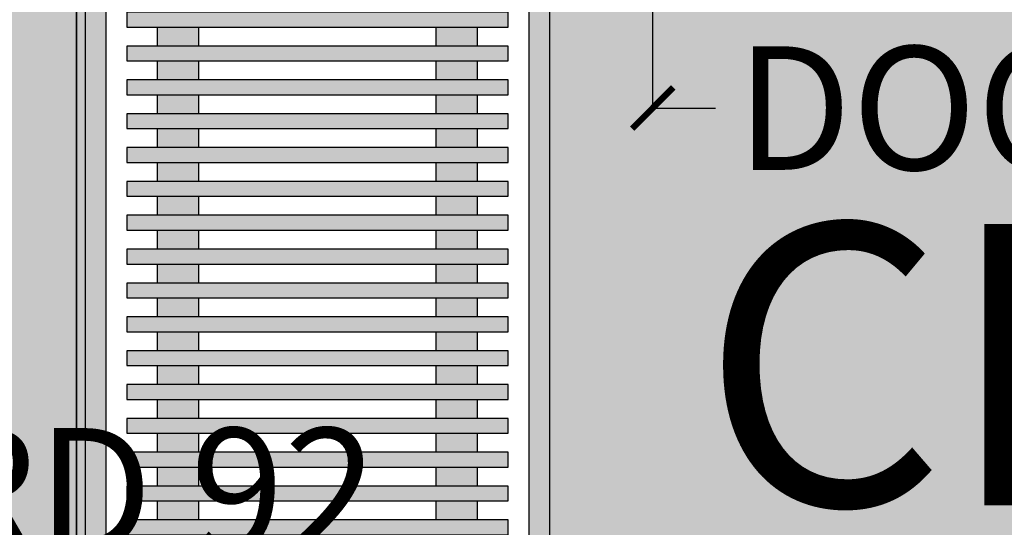
# Model space of a CAD drawing. Units: inches. Extents: x 1704 to 6393, y -157 to 1172.
# Tile 30 of 122: x 2351 to 2398, y 316 to 341. Entities that reach past the tile are written whole.
import ezdxf

# ---------------------------------------------------------------- set-up
doc = ezdxf.new("R2010")
doc.units = ezdxf.units.IN
doc.header["$MEASUREMENT"] = 0
for name, color, linetype, lineweight in [('A-ANNO-DIMS', 7, 'Continuous', 13), ('A-AREA-IDEN', 7, 'Continuous', 18), ('A-FURN', 8, 'Continuous', 18), ('A-WALL-PATT', 7, 'Continuous', 13), ('estofado', 7, 'Continuous', 25), ('WALLS', 7, 'Continuous', 35)]:
    doc.layers.add(name, color=color, linetype=linetype, lineweight=lineweight)
doc.layers.add('A-FLOR-PATT', color=7, linetype='Continuous', lineweight=13, true_color=0xf2f2f2)
doc.layers.add('MOBIL', color=7, linetype='Continuous')
doc.styles.get("Standard").update_dxf_attribs({"font": 'arial.ttf'})
doc.dimstyles.get("Standard").update_dxf_attribs({"dimtxt": 6, "dimasz": 2, "dimexe": 0.18, "dimexo": 0.0625, "dimgap": 0.09, "dimtad": 0, "dimtih": 1, "dimtoh": 1, "dimdec": 1, "dimzin": 0, "dimdsep": 46, "dimlunit": 3, "dimtxsty": 'Standard', "dimblk": 'ARCHTICK', "dimcen": 0.09, "dimadec": 0, "dimazin": 0, "dimtfac": 1, "dimtdec": 1, "dimtofl": 0, "dimtmove": 0, "dimatfit": 3, "dimfxl": 1, "dimtolj": 1, "dimtzin": 0, "dimarcsym": 0})

# ---------------------------------------------------------------- blocks, each defined once
blk = doc.blocks.new('Aparador Aido WV')
at = {"layer": 'MOBIL'}
h = blk.add_hatch(color=256, dxfattribs=at)
h.set_gradient(color1=(226, 228, 228), one_color=1, tint=1, name='CYLINDER')
h.paths.add_polyline_path([(0.9, -0.02), (0.9, 0), (-0.9, 0), (-0.9, -0.02)])
h = blk.add_hatch(color=256, dxfattribs=at)
h.set_gradient(color1=(106, 79, 62), color2=(55, 41, 32), one_color=1, tint=0.17)
h.paths.add_polyline_path([(-0.04342, -0.04017), (-0.04342, -0.40983), (-0.02906, -0.40983), (-0.02906, -0.04017)])
h = blk.add_hatch(color=256, dxfattribs=at)
h.set_gradient(color1=(106, 79, 62), color2=(55, 41, 32), one_color=1, tint=0.17)
h.paths.add_polyline_path([(-0.01067, -0.04017), (-0.01067, -0.40983), (0.00369, -0.40983), (0.00369, -0.04017)])
h = blk.add_hatch(color=256, dxfattribs=at)
h.set_gradient(color1=(106, 79, 62), color2=(55, 41, 32), one_color=1, tint=0.17)
h.paths.add_polyline_path([(0.02208, -0.04017), (0.02208, -0.40983), (0.03644, -0.40983), (0.03644, -0.04017)])
h = blk.add_hatch(color=256, dxfattribs=at)
h.set_gradient(color1=(106, 79, 62), color2=(55, 41, 32), one_color=1, tint=0.17)
h.paths.add_polyline_path([(0.05483, -0.04017), (0.05483, -0.40983), (0.0692, -0.40983), (0.0692, -0.04017)])
h = blk.add_hatch(color=256, dxfattribs=at)
h.set_gradient(color1=(106, 79, 62), color2=(55, 41, 32), one_color=1, tint=0.17)
h.paths.add_polyline_path([(0.10195, -0.04017), (0.08758, -0.04017), (0.08758, -0.40983), (0.10195, -0.40983)])
h = blk.add_hatch(color=256, dxfattribs=at)
h.set_gradient(color1=(106, 79, 62), color2=(55, 41, 32), one_color=1, tint=0.17)
h.paths.add_polyline_path([(0.12033, -0.04017), (0.12033, -0.40983), (0.1347, -0.40983), (0.1347, -0.04017)])
h = blk.add_hatch(color=256, dxfattribs=at)
h.set_gradient(color1=(106, 79, 62), color2=(55, 41, 32), one_color=1, tint=0.17)
h.paths.add_polyline_path([(0.15309, -0.04017), (0.15309, -0.40983), (0.16745, -0.40983), (0.16745, -0.04017)])
h = blk.add_hatch(color=256, dxfattribs=at)
h.set_gradient(color1=(106, 79, 62), color2=(55, 41, 32), one_color=1, tint=0.17)
h.paths.add_polyline_path([(0.18584, -0.04017), (0.18584, -0.40983), (0.2002, -0.40983), (0.2002, -0.04017)])
h = blk.add_hatch(color=256, dxfattribs=at)
h.set_gradient(color1=(106, 79, 62), color2=(55, 41, 32), one_color=1, tint=0.17)
h.paths.add_polyline_path([(0.21859, -0.04017), (0.21859, -0.40983), (0.23295, -0.40983), (0.23295, -0.04017)])
h = blk.add_hatch(color=256, dxfattribs=at)
h.set_gradient(color1=(106, 79, 62), color2=(55, 41, 32), one_color=1, tint=0.17)
h.paths.add_polyline_path([(0.25134, -0.04017), (0.25134, -0.40983), (0.26571, -0.40983), (0.26571, -0.04017)])
h = blk.add_hatch(color=256, dxfattribs=at)
h.set_gradient(color1=(106, 79, 62), color2=(55, 41, 32), one_color=1, tint=0.17)
h.paths.add_polyline_path([(0.28409, -0.04017), (0.28409, -0.40983), (0.29846, -0.40983), (0.29846, -0.04017)])
h = blk.add_hatch(color=256, dxfattribs=at)
h.set_gradient(color1=(106, 79, 62), color2=(55, 41, 32), one_color=1, tint=0.17)
h.paths.add_polyline_path([(0.31684, -0.04017), (0.31684, -0.40983), (0.33121, -0.40983), (0.33121, -0.04017)])
h = blk.add_hatch(color=256, dxfattribs=at)
h.set_gradient(color1=(106, 79, 62), color2=(55, 41, 32), one_color=1, tint=0.17)
h.paths.add_polyline_path([(0.3496, -0.04017), (0.3496, -0.40983), (0.36396, -0.40983), (0.36396, -0.04017)])
h = blk.add_hatch(color=256, dxfattribs=at)
h.set_gradient(color1=(106, 79, 62), color2=(55, 41, 32), one_color=1, tint=0.17)
h.paths.add_polyline_path([(0.38235, -0.04017), (0.38235, -0.40983), (0.39671, -0.40983), (0.39671, -0.04017)])
h = blk.add_hatch(color=256, dxfattribs=at)
h.set_gradient(color1=(106, 79, 62), color2=(55, 41, 32), one_color=1, tint=0.17)
h.paths.add_polyline_path([(0.4151, -0.40983), (0.42946, -0.40983), (0.42946, -0.04017), (0.4151, -0.04017)])
h = blk.add_hatch(color=256, dxfattribs=at)
h.set_gradient(color1=(106, 79, 62), color2=(55, 41, 32), one_color=1, tint=0.17)
h.paths.add_polyline_path([(0.44785, -0.04017), (0.44785, -0.40983), (0.46222, -0.40983), (0.46222, -0.04017)])
h = blk.add_hatch(color=256, dxfattribs=at)
h.set_gradient(color1=(106, 79, 62), color2=(157, 117, 92), one_color=1, tint=0.49)
h.paths.add_polyline_path([(-0.01067, -0.07), (-0.02906, -0.07), (-0.02906, -0.11), (-0.01067, -0.11)])
h = blk.add_hatch(color=256, dxfattribs=at)
h.set_gradient(color1=(106, 79, 62), color2=(157, 117, 92), one_color=1, tint=0.49)
h.paths.add_polyline_path([(0.02208, -0.07), (0.00369, -0.07), (0.00369, -0.11), (0.02208, -0.11)])
h = blk.add_hatch(color=256, dxfattribs=at)
h.set_gradient(color1=(106, 79, 62), color2=(157, 117, 92), one_color=1, tint=0.49)
h.paths.add_polyline_path([(0.05483, -0.07), (0.03644, -0.07), (0.03644, -0.11), (0.05483, -0.11)])
h = blk.add_hatch(color=256, dxfattribs=at)
h.set_gradient(color1=(106, 79, 62), color2=(157, 117, 92), one_color=1, tint=0.49)
h.paths.add_polyline_path([(0.08758, -0.07), (0.0692, -0.07), (0.0692, -0.11), (0.08758, -0.11)])
h = blk.add_hatch(color=256, dxfattribs=at)
h.set_gradient(color1=(106, 79, 62), color2=(157, 117, 92), one_color=1, tint=0.49)
h.paths.add_polyline_path([(0.12033, -0.07), (0.10195, -0.07), (0.10195, -0.11), (0.12033, -0.11)])
h = blk.add_hatch(color=256, dxfattribs=at)
h.set_gradient(color1=(106, 79, 62), color2=(157, 117, 92), one_color=1, tint=0.49)
h.paths.add_polyline_path([(0.15309, -0.07), (0.1347, -0.07), (0.1347, -0.11), (0.15309, -0.11)])
h = blk.add_hatch(color=256, dxfattribs=at)
h.set_gradient(color1=(106, 79, 62), color2=(157, 117, 92), one_color=1, tint=0.49)
h.paths.add_polyline_path([(0.18584, -0.07), (0.16745, -0.07), (0.16745, -0.11), (0.18584, -0.11)])
h = blk.add_hatch(color=256, dxfattribs=at)
h.set_gradient(color1=(106, 79, 62), color2=(157, 117, 92), one_color=1, tint=0.49)
h.paths.add_polyline_path([(0.21859, -0.07), (0.2002, -0.07), (0.2002, -0.11), (0.21859, -0.11)])
h = blk.add_hatch(color=256, dxfattribs=at)
h.set_gradient(color1=(106, 79, 62), color2=(157, 117, 92), one_color=1, tint=0.49)
h.paths.add_polyline_path([(0.25134, -0.07), (0.23295, -0.07), (0.23295, -0.11), (0.25134, -0.11)])
h = blk.add_hatch(color=256, dxfattribs=at)
h.set_gradient(color1=(106, 79, 62), color2=(157, 117, 92), one_color=1, tint=0.49)
h.paths.add_polyline_path([(0.28409, -0.07), (0.26571, -0.07), (0.26571, -0.11), (0.28409, -0.11)])
h = blk.add_hatch(color=256, dxfattribs=at)
h.set_gradient(color1=(106, 79, 62), color2=(157, 117, 92), one_color=1, tint=0.49)
h.paths.add_polyline_path([(0.31684, -0.07), (0.29846, -0.07), (0.29846, -0.11), (0.31684, -0.11)])
h = blk.add_hatch(color=256, dxfattribs=at)
h.set_gradient(color1=(106, 79, 62), color2=(157, 117, 92), one_color=1, tint=0.49)
h.paths.add_polyline_path([(0.3496, -0.07), (0.33121, -0.07), (0.33121, -0.11), (0.3496, -0.11)])
h = blk.add_hatch(color=256, dxfattribs=at)
h.set_gradient(color1=(106, 79, 62), color2=(157, 117, 92), one_color=1, tint=0.49)
h.paths.add_polyline_path([(0.38235, -0.07), (0.36396, -0.07), (0.36396, -0.11), (0.38235, -0.11)])
h = blk.add_hatch(color=256, dxfattribs=at)
h.set_gradient(color1=(106, 79, 62), color2=(157, 117, 92), one_color=1, tint=0.49)
h.paths.add_polyline_path([(0.4151, -0.07), (0.39671, -0.07), (0.39671, -0.11), (0.4151, -0.11)])
h = blk.add_hatch(color=256, dxfattribs=at)
h.set_gradient(color1=(106, 79, 62), color2=(157, 117, 92), one_color=1, tint=0.49)
h.paths.add_polyline_path([(0.44785, -0.07), (0.42946, -0.07), (0.42946, -0.11), (0.44785, -0.11)])
h = blk.add_hatch(color=256, dxfattribs=at)
h.set_gradient(color1=(106, 79, 62), color2=(157, 117, 92), one_color=1, tint=0.49)
h.paths.add_polyline_path([(-0.01067, -0.34), (-0.02906, -0.34), (-0.02906, -0.38), (-0.01067, -0.38)])
h = blk.add_hatch(color=256, dxfattribs=at)
h.set_gradient(color1=(106, 79, 62), color2=(157, 117, 92), one_color=1, tint=0.49)
h.paths.add_polyline_path([(0.02208, -0.34), (0.00369, -0.34), (0.00369, -0.38), (0.02208, -0.38)])
h = blk.add_hatch(color=256, dxfattribs=at)
h.set_gradient(color1=(106, 79, 62), color2=(157, 117, 92), one_color=1, tint=0.49)
h.paths.add_polyline_path([(0.05483, -0.34), (0.03644, -0.34), (0.03644, -0.38), (0.05483, -0.38)])
h = blk.add_hatch(color=256, dxfattribs=at)
h.set_gradient(color1=(106, 79, 62), color2=(157, 117, 92), one_color=1, tint=0.49)
h.paths.add_polyline_path([(0.08758, -0.34), (0.0692, -0.34), (0.0692, -0.38), (0.08758, -0.38)])
h = blk.add_hatch(color=256, dxfattribs=at)
h.set_gradient(color1=(106, 79, 62), color2=(157, 117, 92), one_color=1, tint=0.49)
h.paths.add_polyline_path([(0.12033, -0.34), (0.10195, -0.34), (0.10195, -0.38), (0.12033, -0.38)])
h = blk.add_hatch(color=256, dxfattribs=at)
h.set_gradient(color1=(106, 79, 62), color2=(157, 117, 92), one_color=1, tint=0.49)
h.paths.add_polyline_path([(0.15309, -0.34), (0.1347, -0.34), (0.1347, -0.38), (0.15309, -0.38)])
h = blk.add_hatch(color=256, dxfattribs=at)
h.set_gradient(color1=(106, 79, 62), color2=(157, 117, 92), one_color=1, tint=0.49)
h.paths.add_polyline_path([(0.18584, -0.34), (0.16745, -0.34), (0.16745, -0.38), (0.18584, -0.38)])
h = blk.add_hatch(color=256, dxfattribs=at)
h.set_gradient(color1=(106, 79, 62), color2=(157, 117, 92), one_color=1, tint=0.49)
h.paths.add_polyline_path([(0.21859, -0.34), (0.2002, -0.34), (0.2002, -0.38), (0.21859, -0.38)])
h = blk.add_hatch(color=256, dxfattribs=at)
h.set_gradient(color1=(106, 79, 62), color2=(157, 117, 92), one_color=1, tint=0.49)
h.paths.add_polyline_path([(0.25134, -0.34), (0.23295, -0.34), (0.23295, -0.38), (0.25134, -0.38)])
h = blk.add_hatch(color=256, dxfattribs=at)
h.set_gradient(color1=(106, 79, 62), color2=(157, 117, 92), one_color=1, tint=0.49)
h.paths.add_polyline_path([(0.28409, -0.34), (0.26571, -0.34), (0.26571, -0.38), (0.28409, -0.38)])
h = blk.add_hatch(color=256, dxfattribs=at)
h.set_gradient(color1=(106, 79, 62), color2=(157, 117, 92), one_color=1, tint=0.49)
h.paths.add_polyline_path([(0.31684, -0.34), (0.29846, -0.34), (0.29846, -0.38), (0.31684, -0.38)])
h = blk.add_hatch(color=256, dxfattribs=at)
h.set_gradient(color1=(106, 79, 62), color2=(157, 117, 92), one_color=1, tint=0.49)
h.paths.add_polyline_path([(0.3496, -0.34), (0.33121, -0.34), (0.33121, -0.38), (0.3496, -0.38)])
h = blk.add_hatch(color=256, dxfattribs=at)
h.set_gradient(color1=(106, 79, 62), color2=(157, 117, 92), one_color=1, tint=0.49)
h.paths.add_polyline_path([(0.38235, -0.34), (0.36396, -0.34), (0.36396, -0.38), (0.38235, -0.38)])
h = blk.add_hatch(color=256, dxfattribs=at)
h.set_gradient(color1=(106, 79, 62), color2=(157, 117, 92), one_color=1, tint=0.49)
h.paths.add_polyline_path([(0.4151, -0.34), (0.39671, -0.34), (0.39671, -0.38), (0.4151, -0.38)])
h = blk.add_hatch(color=256, dxfattribs=at)
h.set_gradient(color1=(106, 79, 62), color2=(157, 117, 92), one_color=1, tint=0.49)
h.paths.add_polyline_path([(0.44785, -0.34), (0.42946, -0.34), (0.42946, -0.38), (0.44785, -0.38)])
h = blk.add_hatch(color=256, dxfattribs=at)
h.set_gradient(color1=(226, 228, 228), one_color=1, tint=1, name='CYLINDER')
h.paths.add_polyline_path([(0.9, -0.45), (0.9, -0.43), (-0.9, -0.43), (-0.9, -0.45)])
at = {"layer": 'estofado', "ltscale": 0.5}
for p, q in [((-0.02906, -0.07), (-0.01067, -0.07)), ((0.00369, -0.07), (0.02208, -0.07)), ((0.03644, -0.07), (0.05483, -0.07)), ((0.0692, -0.07), (0.08758, -0.07)), ((0.10195, -0.07), (0.12033, -0.07)), ((0.1347, -0.07), (0.15309, -0.07)), ((0.16745, -0.07), (0.18584, -0.07)), ((0.2002, -0.07), (0.21859, -0.07)), ((0.23295, -0.07), (0.25134, -0.07)), ((0.26571, -0.07), (0.28409, -0.07)), ((0.29846, -0.07), (0.31684, -0.07)), ((0.33121, -0.07), (0.3496, -0.07)), ((0.36396, -0.07), (0.38235, -0.07)), ((0.39671, -0.07), (0.4151, -0.07)), ((0.42946, -0.07), (0.44785, -0.07)), ((-0.02906, -0.11), (-0.01067, -0.11)), ((0.00369, -0.11), (0.02208, -0.11)), ((0.03644, -0.11), (0.05483, -0.11)), ((0.0692, -0.11), (0.08758, -0.11)), ((0.10195, -0.11), (0.12033, -0.11)), ((0.1347, -0.11), (0.15309, -0.11)), ((0.16745, -0.11), (0.18584, -0.11)), ((0.2002, -0.11), (0.21859, -0.11)), ((0.23295, -0.11), (0.25134, -0.11)), ((0.26571, -0.11), (0.28409, -0.11)), ((0.29846, -0.11), (0.31684, -0.11)), ((0.33121, -0.11), (0.3496, -0.11)), ((0.36396, -0.11), (0.38235, -0.11)), ((0.39671, -0.11), (0.4151, -0.11)), ((0.42946, -0.11), (0.44785, -0.11)), ((-0.02906, -0.34), (-0.01067, -0.34)), ((0.00369, -0.34), (0.02208, -0.34)), ((0.03644, -0.34), (0.05483, -0.34)), ((0.0692, -0.34), (0.08758, -0.34)), ((0.10195, -0.34), (0.12033, -0.34)), ((0.1347, -0.34), (0.15309, -0.34)), ((0.16745, -0.34), (0.18584, -0.34)), ((0.2002, -0.34), (0.21859, -0.34)), ((0.23295, -0.34), (0.25134, -0.34)), ((0.26571, -0.34), (0.28409, -0.34)), ((0.29846, -0.34), (0.31684, -0.34)), ((0.33121, -0.34), (0.3496, -0.34)), ((0.36396, -0.34), (0.38235, -0.34)), ((0.39671, -0.34), (0.4151, -0.34)), ((0.42946, -0.34), (0.44785, -0.34)), ((-0.02906, -0.38), (-0.01067, -0.38)), ((0.00369, -0.38), (0.02208, -0.38)), ((0.03644, -0.38), (0.05483, -0.38)), ((0.0692, -0.38), (0.08758, -0.38)), ((0.10195, -0.38), (0.12033, -0.38)), ((0.1347, -0.38), (0.15309, -0.38)), ((0.16745, -0.38), (0.18584, -0.38)), ((0.2002, -0.38), (0.21859, -0.38)), ((0.23295, -0.38), (0.25134, -0.38)), ((0.26571, -0.38), (0.28409, -0.38)), ((0.29846, -0.38), (0.31684, -0.38)), ((0.33121, -0.38), (0.3496, -0.38)), ((0.36396, -0.38), (0.38235, -0.38)), ((0.39671, -0.38), (0.4151, -0.38)), ((0.42946, -0.38), (0.44785, -0.38))]:
    blk.add_line(p, q, dxfattribs=at)
for points in [[(-0.04342, -0.04017), (-0.04342, -0.40983), (-0.02906, -0.40983), (-0.02906, -0.04017)], [(-0.01067, -0.04017), (-0.01067, -0.40983), (0.00369, -0.40983), (0.00369, -0.04017)], [(0.02208, -0.04017), (0.02208, -0.40983), (0.03644, -0.40983), (0.03644, -0.04017)], [(0.05483, -0.04017), (0.05483, -0.40983), (0.0692, -0.40983), (0.0692, -0.04017)], [(0.08758, -0.04017), (0.08758, -0.40983), (0.10195, -0.40983), (0.10195, -0.04017)], [(0.12033, -0.04017), (0.12033, -0.40983), (0.1347, -0.40983), (0.1347, -0.04017)], [(0.15309, -0.04017), (0.15309, -0.40983), (0.16745, -0.40983), (0.16745, -0.04017)], [(0.18584, -0.04017), (0.18584, -0.40983), (0.2002, -0.40983), (0.2002, -0.04017)], [(0.21859, -0.04017), (0.21859, -0.40983), (0.23295, -0.40983), (0.23295, -0.04017)], [(0.25134, -0.04017), (0.25134, -0.40983), (0.26571, -0.40983), (0.26571, -0.04017)], [(0.28409, -0.04017), (0.28409, -0.40983), (0.29846, -0.40983), (0.29846, -0.04017)], [(0.31684, -0.04017), (0.31684, -0.40983), (0.33121, -0.40983), (0.33121, -0.04017)], [(0.3496, -0.04017), (0.3496, -0.40983), (0.36396, -0.40983), (0.36396, -0.04017)], [(0.38235, -0.04017), (0.38235, -0.40983), (0.39671, -0.40983), (0.39671, -0.04017)], [(0.4151, -0.04017), (0.4151, -0.40983), (0.42946, -0.40983), (0.42946, -0.04017)], [(0.44785, -0.04017), (0.44785, -0.40983), (0.46222, -0.40983), (0.46222, -0.04017)]]:
    blk.add_lwpolyline(points, close=True, dxfattribs=at)
at = {"layer": 'MOBIL'}
for p, q in [((0.9, -0.02), (-0.9, -0.02)), ((-0.9, -0.43), (0.9, -0.43))]:
    blk.add_line(p, q, dxfattribs=at)
blk.add_lwpolyline([(-0.9, -0.45), (0.9, -0.45), (0.9, 0), (-0.9, 0)], close=True, dxfattribs=at)
blk = doc.blocks.new('_ArchTick')
at = {"color": 0, "linetype": 'ByBlock', "const_width": 0.15}
blk.add_lwpolyline([(-0.5, -0.5), (0.5, 0.5)], dxfattribs=at)
blk = doc.blocks.new('*D30')
at = {"layer": 'A-ANNO-DIMS', "color": 0, "lineweight": -2, "transparency": 16777216}
for p, q in [((2381.349, 342.693), (2381.349, 336.276)), ((2423.349, 342.693), (2423.349, 336.276)), ((2381.349, 336.456), (2384.404, 336.456)), ((2423.349, 336.456), (2420.293, 336.456))]:
    blk.add_line(p, q, dxfattribs=at)
at = {"layer": 'Defpoints', "color": 0, "lineweight": -3, "transparency": 16777216}
for p in [(2381.349, 342.756), (2423.349, 342.756), (2423.349, 336.456)]:
    blk.add_point(p, dxfattribs=at)
at = {"layer": 'A-ANNO-DIMS', "color": 0, "lineweight": -2, "transparency": 16777216, "xscale": 2, "yscale": 2, "zscale": 2, "rotation": 180}
blk.add_blockref('_ArchTick', (2381.349, 336.456), dxfattribs=at)
at = {"layer": 'A-ANNO-DIMS', "color": 0, "lineweight": -2, "transparency": 16777216, "xscale": 2, "yscale": 2, "zscale": 2}
blk.add_blockref('_ArchTick', (2423.349, 336.456), dxfattribs=at)
at = {"layer": 'A-ANNO-DIMS', "color": 0, "transparency": 16777216, "insert": (2402.349, 336.456), "char_height": 6, "attachment_point": 5}
blk.add_mtext('\\A1;DOOR 42', dxfattribs=at)
blk = doc.blocks.new('*D68')
at = {"layer": 'A-ANNO-DIMS', "color": 0, "lineweight": -2, "transparency": 16777216}
for p, q in [((2353.706, 363.767), (2339.834, 363.767)), ((2340.014, 363.767), (2340.014, 321.111)), ((2340.014, 272.066), (2340.014, 314.722)), ((2353.706, 272.066), (2339.834, 272.066))]:
    blk.add_line(p, q, dxfattribs=at)
at = {"layer": 'Defpoints', "color": 0, "lineweight": -3, "transparency": 16777216}
for p in [(2340.014, 363.767), (2353.769, 363.767), (2353.769, 272.066)]:
    blk.add_point(p, dxfattribs=at)
at = {"layer": 'A-ANNO-DIMS', "color": 0, "lineweight": -2, "transparency": 16777216, "xscale": 2, "yscale": 2, "zscale": 2}
for p, rotation in [((2340.014, 363.767), 90), ((2340.014, 272.066), 270)]:
    blk.add_blockref('_ArchTick', p, dxfattribs=dict(at, rotation=rotation))
at = {"layer": 'A-ANNO-DIMS', "color": 0, "transparency": 16777216, "insert": (2340.014, 317.916), "char_height": 6, "attachment_point": 5}
blk.add_mtext('\\A1;SIDEBOARD 92', dxfattribs=at)
blk = doc.blocks.new('*D93')
at = {"layer": 'A-ANNO-DIMS', "color": 0, "lineweight": -2, "transparency": 16777216}
for p, q in [((2605.286, 895.213), (1829.698, 895.213)), ((1829.878, 895.213), (1829.878, 495.866)), ((1829.878, 90.213), (1829.878, 489.56)), ((2605.286, 90.213), (1829.698, 90.213))]:
    blk.add_line(p, q, dxfattribs=at)
at = {"layer": 'Defpoints', "color": 0, "lineweight": -3, "transparency": 16777216}
for p in [(2605.349, 895.213), (1829.878, 90.213), (2605.349, 90.213)]:
    blk.add_point(p, dxfattribs=at)
at = {"layer": 'A-ANNO-DIMS', "color": 0, "lineweight": -2, "transparency": 16777216, "xscale": 2, "yscale": 2, "zscale": 2}
for p, rotation in [((1829.878, 895.213), 90), ((1829.878, 90.213), 270)]:
    blk.add_blockref('_ArchTick', p, dxfattribs=dict(at, rotation=rotation))
at = {"layer": 'A-ANNO-DIMS', "color": 0, "transparency": 16777216, "insert": (1829.878, 492.713), "char_height": 6, "attachment_point": 5}
blk.add_mtext('\\A1;805', dxfattribs=at)

msp = doc.modelspace()

# ---------------------------------------------------------------- hatches: boundary and pattern name
at = {"layer": 'A-FLOR-PATT', "transparency": 33554528}
h = msp.add_hatch(color=256, dxfattribs=at)
h.dxf.hatch_style = 1
h.paths.add_polyline_path([(2325.349, 863.213), (2325.349, 887.213), (2263.349, 887.213), (2167.349, 887.213), (2081.349, 887.213), (2081.349, 719.213), (2277.349, 719.213), (2277.349, 711.213), (2277.349, 372.213), (2349.349, 372.213), (2381.349, 372.213), (2381.349, 364.213), (2353.349, 364.213), (2353.349, 270.213), (2381.349, 270.213), (2381.349, 266.213), (2357.349, 266.213), (2357.349, 98.213), (2381.349, 98.213), (2385.181, 98.213), (2386.482, 98.213), (2424.215, 98.213), (2425.516, 98.213), (2429.349, 98.213), (2597.349, 98.213), (2597.349, 146.213), (2597.349, 218.213), (2597.349, 266.213), (2423.349, 266.213), (2423.349, 270.213), (2473.349, 270.213), (2473.349, 294.213), (2477.349, 294.213), (2477.349, 270.213), (2547.349, 270.213), (2547.349, 364.213), (2477.349, 364.213), (2477.349, 318.213), (2473.349, 318.213), (2473.349, 364.213), (2423.349, 364.213), (2423.349, 372.213), (2469.349, 372.213), (2469.349, 459.213), (2469.349, 538.213), (2350.349, 538.213), (2350.349, 565.713), (2358.349, 565.713), (2358.349, 545.213), (2420.349, 545.213), (2420.349, 610.213), (2358.349, 610.213), (2358.349, 589.713), (2350.349, 589.713), (2350.349, 615.213), (2425.349, 615.213), (2425.349, 607.213), (2425.349, 546.213), (2469.349, 546.213), (2514.349, 546.213), (2514.349, 607.213), (2449.349, 607.213), (2449.349, 615.213), (2451.738, 615.213), (2451.738, 659.213), (2427.738, 659.213), (2427.738, 665.213), (2367.738, 665.213), (2367.738, 667.213), (2367.738, 711.213), (2325.349, 711.213), (2325.349, 719.213), (2325.349, 755.213), (2325.349, 763.213)])
h.paths.add_polyline_path([(2233.858, 822.533, -0.187247), (2233.858, 809.14), (2231.697, 808.804, 0.084893), (2233.131, 814.486), (2230.424, 814.486, -0.104258), (2228.553, 808.313), (2217.751, 807.156, -0.222222), (2217.751, 824.517), (2228.553, 823.359, -0.104258), (2230.424, 817.186), (2233.131, 817.186, 0.084893), (2231.697, 822.868)], flags=16)
h.paths.add_polyline_path([(2213.621, 833.197), (2213.621, 798.475), (2156.048, 798.475), (2156.048, 833.197)], flags=16)
h.paths.add_polyline_path([(2203.932, 848.099), (2205.089, 837.296, -0.222222), (2187.728, 837.296), (2188.885, 848.099, -0.104258), (2195.058, 849.969), (2195.058, 852.676, 0.084893), (2189.377, 851.242), (2189.712, 853.404, -0.187247), (2203.105, 853.404), (2203.44, 851.242, 0.084893), (2197.759, 852.676), (2197.759, 849.969, -0.104258)], flags=16)
h.paths.add_polyline_path([(2181.941, 837.296, -0.222222), (2164.58, 837.296), (2165.737, 848.099, -0.104258), (2171.91, 849.969), (2171.91, 852.676, 0.084893), (2166.229, 851.242), (2166.564, 853.404, -0.187247), (2179.957, 853.404), (2180.292, 851.242, 0.084893), (2174.611, 852.676), (2174.611, 849.969, -0.104258), (2180.784, 848.099)], flags=16)
h.paths.add_polyline_path([(2205.089, 794.376), (2203.932, 783.574, -0.104258), (2197.759, 781.703), (2197.759, 778.996, 0.084893), (2203.44, 780.43), (2203.105, 778.269, -0.187247), (2189.712, 778.269), (2189.377, 780.43, 0.084893), (2195.058, 778.996), (2195.058, 781.703, -0.104258), (2188.885, 783.574), (2187.728, 794.376, -0.222222)], flags=16)
h.paths.add_polyline_path([(2181.941, 794.376), (2180.784, 783.574, -0.104258), (2174.611, 781.703), (2174.611, 778.996, 0.084893), (2180.292, 780.43), (2179.957, 778.269, -0.187247), (2166.564, 778.269), (2166.229, 780.43, 0.084893), (2171.91, 778.996), (2171.91, 781.703, -0.104258), (2165.737, 783.574), (2164.58, 794.376, -0.222222)], flags=16)
h.paths.add_polyline_path([(2151.918, 807.156), (2141.116, 808.313, -0.104258), (2139.245, 814.486), (2136.539, 814.486, 0.084893), (2137.972, 808.804), (2135.811, 809.14, -0.187247), (2135.811, 822.533), (2137.972, 822.868, 0.084893), (2136.539, 817.186), (2139.245, 817.186, -0.104258), (2141.116, 823.359), (2151.918, 824.517, -0.222222)], flags=16)
h.paths.add_polyline_path([(2357.868, 363.41), (2358.814, 363.41, 0.75376)], flags=16)
h.paths.add_polyline_path([(2372.241, 363.117), (2372.248, 363.117), (2372.248, 363.343), (2371.302, 363.343), (2371.302, 363.139, -1.360391)], flags=16)
h.paths.add_polyline_path([(2371.309, 272.716), (2371.302, 272.716), (2371.302, 272.49), (2372.248, 272.49), (2372.248, 272.693, -1.360391)], flags=16)
h.paths.add_polyline_path([(2357.875, 272.716), (2357.868, 272.716), (2357.868, 272.49), (2358.814, 272.49), (2358.814, 272.693, -1.360391)], flags=16)
h.paths.add_polyline_path([(2353.769, 363.074), (2376.347, 363.074), (2376.347, 272.759), (2353.769, 272.759)], flags=16)
h.paths.add_polyline_path([(2354.772, 362.07), (2375.344, 362.07), (2375.344, 273.762), (2354.772, 273.762)], flags=0)
h.paths.add_polyline_path([(2357.868, 363.343), (2358.814, 363.343), (2358.814, 363.117), (2357.868, 363.117)], flags=16)
h.paths.add_polyline_path([(2359.288, 359.184), (2359.288, 360.063), (2370.828, 360.063), (2370.828, 359.184), (2374.332, 359.184), (2374.332, 358.464), (2372.835, 358.464), (2372.835, 357.541), (2374.332, 357.541), (2374.332, 356.82), (2372.835, 356.82), (2372.835, 355.898), (2374.332, 355.898), (2374.332, 355.177), (2372.835, 355.177), (2372.835, 354.254), (2374.332, 354.254), (2374.332, 353.534), (2372.835, 353.534), (2372.835, 352.611), (2374.332, 352.611), (2374.332, 351.89), (2372.835, 351.89), (2372.835, 350.968), (2374.332, 350.968), (2374.332, 350.247), (2372.835, 350.247), (2372.835, 349.324), (2374.332, 349.324), (2374.332, 348.604), (2372.835, 348.604), (2372.835, 347.681), (2374.332, 347.681), (2374.332, 346.96), (2372.835, 346.96), (2372.835, 346.038), (2374.332, 346.038), (2374.332, 345.317), (2372.835, 345.317), (2372.835, 344.395), (2374.332, 344.395), (2374.332, 343.674), (2372.835, 343.674), (2372.835, 342.751), (2374.332, 342.751), (2374.332, 342.03), (2372.835, 342.03), (2372.835, 341.108), (2374.332, 341.108), (2374.332, 340.387), (2372.835, 340.387), (2372.835, 339.465), (2374.332, 339.465), (2374.332, 338.744), (2372.835, 338.744), (2372.835, 337.821), (2374.332, 337.821), (2374.332, 337.1), (2372.835, 337.1), (2372.835, 336.178), (2374.332, 336.178), (2374.332, 335.457), (2372.835, 335.457), (2372.835, 334.535), (2374.332, 334.535), (2374.332, 333.814), (2372.835, 333.814), (2372.835, 332.891), (2374.332, 332.891), (2374.332, 332.171), (2372.835, 332.171), (2372.835, 331.248), (2374.332, 331.248), (2374.332, 330.527), (2372.835, 330.527), (2372.835, 329.605), (2374.332, 329.605), (2374.332, 328.884), (2372.835, 328.884), (2372.835, 327.961), (2374.332, 327.961), (2374.332, 327.241), (2372.835, 327.241), (2372.835, 326.318), (2374.332, 326.318), (2374.332, 325.597), (2372.835, 325.597), (2372.835, 324.675), (2374.332, 324.675), (2374.332, 323.954), (2372.835, 323.954), (2372.835, 323.031), (2374.332, 323.031), (2374.332, 322.311), (2372.835, 322.311), (2372.835, 321.388), (2374.332, 321.388), (2374.332, 320.667), (2372.835, 320.667), (2372.835, 319.745), (2374.332, 319.745), (2374.332, 319.024), (2372.835, 319.024), (2372.835, 318.102), (2374.332, 318.102), (2374.332, 317.381), (2372.835, 317.381), (2372.835, 316.458), (2374.332, 316.458), (2374.332, 315.737), (2372.835, 315.737), (2372.835, 314.815), (2374.332, 314.815), (2374.332, 314.094), (2372.835, 314.094), (2372.835, 313.172), (2374.332, 313.172), (2374.332, 312.451), (2372.835, 312.451), (2372.835, 311.528), (2374.332, 311.528), (2374.332, 310.807), (2372.835, 310.807), (2372.835, 309.885), (2374.332, 309.885), (2374.332, 309.164), (2372.835, 309.164), (2372.835, 308.242), (2374.332, 308.242), (2374.332, 307.521), (2372.835, 307.521), (2372.835, 306.598), (2374.332, 306.598), (2374.332, 305.878), (2372.835, 305.878), (2372.835, 304.955), (2374.332, 304.955), (2374.332, 304.234), (2372.835, 304.234), (2372.835, 303.312), (2374.332, 303.312), (2374.332, 302.591), (2372.835, 302.591), (2372.835, 301.668), (2374.332, 301.668), (2374.332, 300.948), (2372.835, 300.948), (2372.835, 300.025), (2374.332, 300.025), (2374.332, 299.304), (2372.835, 299.304), (2372.835, 298.382), (2374.332, 298.382), (2374.332, 297.661), (2372.835, 297.661), (2372.835, 296.738), (2374.332, 296.738), (2374.332, 296.018), (2372.835, 296.018), (2372.835, 295.095), (2374.332, 295.095), (2374.332, 294.374), (2372.835, 294.374), (2372.835, 293.452), (2374.332, 293.452), (2374.332, 292.731), (2372.835, 292.731), (2372.835, 291.809), (2374.332, 291.809), (2374.332, 291.088), (2372.835, 291.088), (2372.835, 290.165), (2374.332, 290.165), (2374.332, 289.444), (2372.835, 289.444), (2372.835, 288.522), (2374.332, 288.522), (2374.332, 287.801), (2372.835, 287.801), (2372.835, 286.879), (2374.332, 286.879), (2374.332, 286.158), (2372.835, 286.158), (2372.835, 285.235), (2374.332, 285.235), (2374.332, 284.514), (2372.835, 284.514), (2372.835, 283.592), (2374.332, 283.592), (2374.332, 282.871), (2372.835, 282.871), (2372.835, 281.949), (2374.332, 281.949), (2374.332, 281.228), (2372.835, 281.228), (2372.835, 280.305), (2374.332, 280.305), (2374.332, 279.585), (2372.835, 279.585), (2372.835, 278.662), (2374.332, 278.662), (2374.332, 277.941), (2372.835, 277.941), (2372.835, 277.019), (2374.332, 277.019), (2374.332, 276.298), (2370.828, 276.298), (2370.828, 275.769), (2359.288, 275.769), (2359.288, 276.298), (2355.784, 276.298), (2355.784, 277.019), (2357.281, 277.019), (2357.281, 277.941), (2355.784, 277.941), (2355.784, 278.662), (2357.281, 278.662), (2357.281, 279.585), (2355.784, 279.585), (2355.784, 280.305), (2357.281, 280.305), (2357.281, 281.228), (2355.784, 281.228), (2355.784, 281.949), (2357.281, 281.949), (2357.281, 282.871), (2355.784, 282.871), (2355.784, 283.592), (2357.281, 283.592), (2357.281, 284.514), (2355.784, 284.514), (2355.784, 285.235), (2357.281, 285.235), (2357.281, 286.158), (2355.784, 286.158), (2355.784, 286.879), (2357.281, 286.879), (2357.281, 287.801), (2355.784, 287.801), (2355.784, 288.522), (2357.281, 288.522), (2357.281, 289.444), (2355.784, 289.444), (2355.784, 290.165), (2357.281, 290.165), (2357.281, 291.088), (2355.784, 291.088), (2355.784, 291.809), (2357.281, 291.809), (2357.281, 292.731), (2355.784, 292.731), (2355.784, 293.452), (2357.281, 293.452), (2357.281, 294.374), (2355.784, 294.374), (2355.784, 295.095), (2357.281, 295.095), (2357.281, 296.018), (2355.784, 296.018), (2355.784, 296.738), (2357.281, 296.738), (2357.281, 297.661), (2355.784, 297.661), (2355.784, 298.382), (2357.281, 298.382), (2357.281, 299.304), (2355.784, 299.304), (2355.784, 300.025), (2357.281, 300.025), (2357.281, 300.948), (2355.784, 300.948), (2355.784, 301.668), (2357.281, 301.668), (2357.281, 302.591), (2355.784, 302.591), (2355.784, 303.312), (2357.281, 303.312), (2357.281, 304.234), (2355.784, 304.234), (2355.784, 304.955), (2357.281, 304.955), (2357.281, 305.878), (2355.784, 305.878), (2355.784, 306.598), (2357.281, 306.598), (2357.281, 307.521), (2355.784, 307.521), (2355.784, 308.242), (2357.281, 308.242), (2357.281, 309.164), (2355.784, 309.164), (2355.784, 309.885), (2357.281, 309.885), (2357.281, 310.807), (2355.784, 310.807), (2355.784, 311.528), (2357.281, 311.528), (2357.281, 312.451), (2355.784, 312.451), (2355.784, 313.172), (2357.281, 313.172), (2357.281, 314.094), (2355.784, 314.094), (2355.784, 314.815), (2357.281, 314.815), (2357.281, 315.737), (2355.784, 315.737), (2355.784, 316.458), (2357.281, 316.458), (2357.281, 317.381), (2355.784, 317.381), (2355.784, 318.102), (2357.281, 318.102), (2357.281, 319.024), (2355.784, 319.024), (2355.784, 319.745), (2357.281, 319.745), (2357.281, 320.667), (2355.784, 320.667), (2355.784, 321.388), (2357.281, 321.388), (2357.281, 322.311), (2355.784, 322.311), (2355.784, 323.031), (2357.281, 323.031), (2357.281, 323.954), (2355.784, 323.954), (2355.784, 324.675), (2357.281, 324.675), (2357.281, 325.597), (2355.784, 325.597), (2355.784, 326.318), (2357.281, 326.318), (2357.281, 327.241), (2355.784, 327.241), (2355.784, 327.961), (2357.281, 327.961), (2357.281, 328.884), (2355.784, 328.884), (2355.784, 329.605), (2357.281, 329.605), (2357.281, 330.527), (2355.784, 330.527), (2355.784, 331.248), (2357.281, 331.248), (2357.281, 332.171), (2355.784, 332.171), (2355.784, 332.891), (2357.281, 332.891), (2357.281, 333.814), (2355.784, 333.814), (2355.784, 334.535), (2357.281, 334.535), (2357.281, 335.457), (2355.784, 335.457), (2355.784, 336.178), (2357.281, 336.178), (2357.281, 337.1), (2355.784, 337.1), (2355.784, 337.821), (2357.281, 337.821), (2357.281, 338.744), (2355.784, 338.744), (2355.784, 339.465), (2357.281, 339.465), (2357.281, 340.387), (2355.784, 340.387), (2355.784, 341.108), (2357.281, 341.108), (2357.281, 342.03), (2355.784, 342.03), (2355.784, 342.751), (2357.281, 342.751), (2357.281, 343.674), (2355.784, 343.674), (2355.784, 344.395), (2357.281, 344.395), (2357.281, 345.317), (2355.784, 345.317), (2355.784, 346.038), (2357.281, 346.038), (2357.281, 346.96), (2355.784, 346.96), (2355.784, 347.681), (2357.281, 347.681), (2357.281, 348.604), (2355.784, 348.604), (2355.784, 349.324), (2357.281, 349.324), (2357.281, 350.247), (2355.784, 350.247), (2355.784, 350.968), (2357.281, 350.968), (2357.281, 351.89), (2355.784, 351.89), (2355.784, 352.611), (2357.281, 352.611), (2357.281, 353.534), (2355.784, 353.534), (2355.784, 354.254), (2357.281, 354.254), (2357.281, 355.177), (2355.784, 355.177), (2355.784, 355.898), (2357.281, 355.898), (2357.281, 356.82), (2355.784, 356.82), (2355.784, 357.541), (2357.281, 357.541), (2357.281, 358.464), (2355.784, 358.464), (2355.784, 359.184)], flags=0)
at = {"layer": 'A-WALL-PATT', "transparency": 33554643}
h = msp.add_hatch(color=256, dxfattribs=at)
h.dxf.hatch_style = 1
h.paths.add_polyline_path([(2167.349, 895.213), (2073.349, 895.213), (2073.349, 887.213), (2081.349, 887.213), (2167.349, 887.213)])
h.paths.add_polyline_path([(2465.349, 895.213), (2273.349, 895.213), (2273.349, 903.213), (2263.349, 903.213), (2263.349, 895.213), (2263.349, 887.213), (2325.349, 887.213), (2325.349, 863.213), (2333.349, 863.213), (2333.349, 887.213), (2465.349, 887.213)])
h.paths.add_polyline_path([(2533.349, 895.213), (2513.349, 895.213), (2513.349, 887.213), (2513.349, 861.213), (2517.349, 861.213), (2517.349, 887.213), (2533.349, 887.213)])
h.paths.add_polyline_path([(2605.349, 895.213), (2581.349, 895.213), (2581.349, 887.213), (2597.349, 887.213), (2597.349, 854.213), (2605.349, 854.213)])
h.paths.add_polyline_path([(2605.349, 752.213), (2629.349, 752.213), (2629.349, 716.213), (2605.349, 716.213), (2605.349, 712.213), (2719.349, 712.213), (2719.349, 716.213), (2631.349, 716.213), (2631.349, 754.213), (2605.349, 754.213), (2605.349, 794.213), (2597.349, 794.213), (2597.349, 787.213), (2517.349, 787.213), (2517.349, 813.213), (2513.349, 813.213), (2513.349, 783.213), (2517.349, 783.213), (2597.349, 783.213), (2597.349, 719.213), (2517.349, 719.213), (2517.349, 753.213), (2513.349, 753.213), (2513.349, 719.213), (2365.349, 719.213), (2365.349, 763.213), (2325.349, 763.213), (2325.349, 755.213), (2357.349, 755.213), (2357.349, 719.213), (2325.349, 719.213), (2325.349, 711.213), (2547.349, 711.213), (2547.349, 615.213), (2449.349, 615.213), (2449.349, 607.213), (2514.349, 607.213), (2514.349, 546.213), (2439.349, 546.213), (2425.349, 546.213), (2425.349, 607.213), (2425.349, 615.213), (2350.349, 615.213), (2350.349, 589.713), (2358.349, 589.713), (2358.349, 610.213), (2420.349, 610.213), (2420.349, 545.213), (2358.349, 545.213), (2358.349, 565.713), (2350.349, 565.713), (2350.349, 538.213), (2469.349, 538.213), (2469.349, 459.213), (2469.349, 372.213), (2423.349, 372.213), (2423.349, 364.213), (2473.349, 364.213), (2473.349, 318.213), (2477.349, 318.213), (2477.349, 364.213), (2547.349, 364.213), (2547.349, 352.213), (2549.349, 352.213), (2549.349, 364.213), (2597.349, 364.213), (2597.349, 328.213), (2549.349, 328.213), (2547.349, 328.213), (2547.349, 326.213), (2549.349, 326.213), (2597.349, 326.213), (2605.349, 326.213), (2605.349, 377.057), (2597.349, 377.057), (2597.349, 372.213), (2477.349, 372.213), (2477.349, 451.213), (2597.349, 451.213), (2605.349, 451.213), (2605.349, 459.213), (2597.349, 459.213), (2477.349, 459.213), (2477.349, 538.213), (2597.349, 538.213), (2597.349, 495.213), (2605.349, 495.213), (2605.349, 512.213), (2631.349, 512.213), (2631.349, 568.213), (2605.349, 568.213), (2605.349, 577.213), (2597.349, 577.213), (2597.349, 542.213), (2518.349, 542.213), (2518.349, 607.213), (2532.349, 607.213), (2605.349, 607.213), (2605.349, 615.213), (2597.349, 615.213), (2551.349, 615.213), (2551.349, 711.213), (2597.349, 711.213), (2597.349, 645.213), (2605.349, 645.213), (2605.349, 712.213), (2605.349, 716.213)])
h.paths.add_polyline_path([(2605.349, 566.213), (2629.349, 566.213), (2629.349, 514.213), (2605.349, 514.213)], flags=16)
h.paths.add_polyline_path([(2381.349, 372.213), (2349.349, 372.213), (2349.349, 202.213), (2337.349, 202.213), (2337.349, 194.213), (2349.349, 194.213), (2349.349, 90.213), (2349.349, 72.213), (2357.349, 72.213), (2357.349, 90.213), (2381.349, 90.213), (2381.349, 98.213), (2357.349, 98.213), (2357.349, 266.213), (2381.349, 266.213), (2381.349, 270.213), (2353.349, 270.213), (2353.349, 364.213), (2381.349, 364.213)])
h.paths.add_polyline_path([(2605.349, 302.213), (2597.349, 302.213), (2597.349, 270.213), (2477.349, 270.213), (2477.349, 294.213), (2473.349, 294.213), (2473.349, 270.213), (2423.349, 270.213), (2423.349, 266.213), (2597.349, 266.213), (2597.349, 218.213), (2605.349, 218.213)])
h.paths.add_polyline_path([(2605.349, 146.213), (2597.349, 146.213), (2597.349, 98.213), (2429.349, 98.213), (2429.349, 90.213), (2597.349, 90.213), (2597.349, 72.213), (2605.349, 72.213), (2605.349, 90.213)])
h.paths.add_polyline_path([(2225.349, 202.213), (2049.349, 202.213), (2049.349, 194.213), (2225.349, 194.213)])
h.paths.add_polyline_path([(2289.349, 202.213), (2277.349, 202.213), (2273.349, 202.213), (2269.516, 202.213), (2269.516, 194.213), (2273.349, 194.213), (2277.349, 194.213), (2289.349, 194.213)])
h.paths.add_polyline_path([(2273.349, 372.213), (2029.19, 372.213), (2029.19, 364.213), (2273.349, 364.213)])
h.paths.add_polyline_path([(2277.349, 545.213), (2213.349, 545.213), (2213.349, 573.213), (2205.349, 573.213), (2177.349, 573.213), (2177.349, 545.213), (2073.349, 545.213), (2073.349, 538.213), (2081.349, 538.213), (2277.349, 538.213)])
h.paths.add_polyline_path([(2181.349, 545.213), (2181.349, 569.213), (2205.349, 569.213), (2205.349, 545.213)], flags=16)
h.paths.add_polyline_path([(2277.349, 719.213), (2081.349, 719.213), (2073.349, 719.213), (2073.349, 711.213), (2154.575, 711.213), (2205.349, 711.213), (2205.349, 687.213), (2205.349, 629.213), (2213.349, 629.213), (2273.349, 629.213), (2273.349, 631.213), (2207.349, 631.213), (2207.349, 707.213), (2231.349, 707.213), (2231.349, 709.213), (2207.349, 709.213), (2207.349, 711.213), (2277.349, 711.213)])

# ---------------------------------------------------------------- linework, layer by layer
at = {"layer": 'WALLS'}
msp.add_line((2353.349, 270.213), (2353.349, 364.213), dxfattribs=at)

# ---------------------------------------------------------------- block references
at = {"layer": 'A-FURN', "xscale": 50.174952135231, "yscale": 50.174952135231, "zscale": 50.174952135231, "rotation": 90}
msp.add_blockref('Aparador Aido WV', (2353.769, 317.916), dxfattribs=at)

# ---------------------------------------------------------------- texts
at = {"layer": 'A-AREA-IDEN'}
msp.add_text('CLOSET', height=13.6672, dxfattribs=at).set_placement((2383.693, 317.16))

# ---------------------------------------------------------------- dimensions: what is measured, and where the dimension line sits
at = {"layer": 'A-ANNO-DIMS'}
dim = msp.add_linear_dim(base=(1829.878, 90.213), p1=(2605.349, 895.213), p2=(2605.349, 90.213), angle=90, dimstyle='Standard', override={"dimdec": 0, "dimlfac": 1, "dimrnd": 0, "dimzin": 0, "dimdsep": 46, "dimlunit": 2}, dxfattribs=at)
dim.commit()
dim.dimension.update_dxf_attribs({"geometry": '*D93', "text_midpoint": (1829.878, 492.713)})
dim = msp.add_linear_dim(base=(2340.014, 363.767), p1=(2353.769, 272.066), p2=(2353.769, 363.767), angle=90, text='SIDEBOARD <>', dimstyle='Standard', override={"dimdec": 0, "dimlfac": 1, "dimrnd": 0, "dimzin": 0, "dimdsep": 46, "dimlunit": 2}, dxfattribs=at)
dim.commit()
dim.dimension.update_dxf_attribs({"geometry": '*D68', "text_midpoint": (2340.014, 317.916)})
dim = msp.add_linear_dim(base=(2423.349, 336.456), p1=(2381.349, 342.756), p2=(2423.349, 342.756), text='DOOR <>', dimstyle='Standard', override={"dimdec": 0, "dimlfac": 1, "dimrnd": 0, "dimzin": 0, "dimdsep": 46, "dimlunit": 2}, dxfattribs=at)
dim.commit()
dim.dimension.update_dxf_attribs({"geometry": '*D30', "text_midpoint": (2402.349, 336.456)})

doc.saveas('drawing.dxf')
